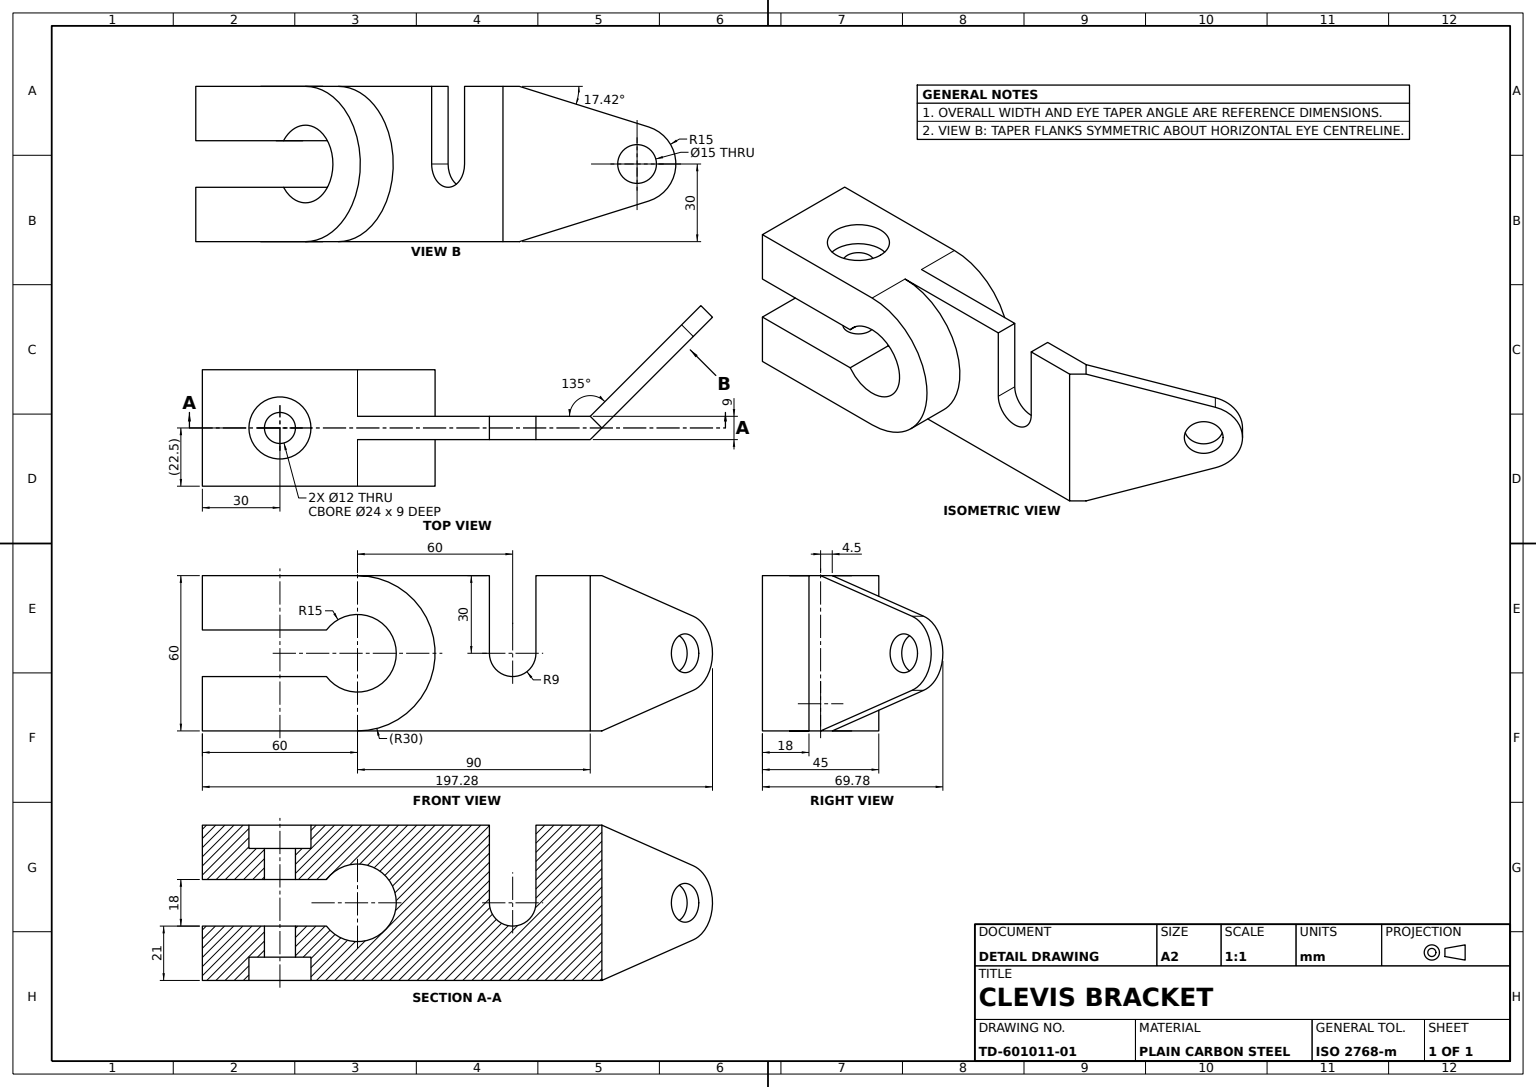
SolidWorks part; units mm, degrees
material "Plain Carbon Steel"
ref_plane "Front Plane" through (0, 0, 0) normal (0, 0, 1) x (1, 0, 0)
ref_plane "Top Plane" through (0, 0, 0) normal (0, 1, 0) x (1, 0, 0)
ref_plane "Right Plane" through (0, 0, 0) normal (1, 0, 0) x (0, 0, -1)
sketch "Clevis Block Sketch" plane through (0, 0, 0) normal (0, 0, 1) x (1, 0, 0)
  line L0 (0, -30) -> (-60, -30)
  line L5 (-60, -30) -> (-60, -9)
  line L6 (0, 30) -> (-60, 30)
  line L7 (0, 0) -> (-30, 0)
  line L8 (-12, 9) -> (-28.6182, 9)
  line L9 (-12, -9) -> (-28.6182, -9)
  line L10 (0, 9) -> (-30, 9) construction
  line L11 (0, -9) -> (-30, -9) construction
  line L12 (-28.6182, 9) -> (-60, 9)
  line L13 (-28.6182, -9) -> (-60, -9)
  line L14 (-60, 9) -> (-60, 30)
  arc A0 (-12, -9) -> (-12, 9) centre (0, 0) ccw
  arc A1 (0, -30) -> (0, 30) centre (0, 0) ccw
  dimension "D1" = 30
  dimension "D2" = 60
  dimension "D3" = 60
  dimension "D6" = 30
  dimension "D7" = 28.6182
  dimension "D4" = 9
  dimension "D5" = 9
extrude "Clevis Block" add sketch "Clevis Block Sketch" along normal mid plane 45 contours L0 A1 L6 L14 L12 L8 A0 L9 L13 L5
sketch "Counterbore Sketch" plane through (0, 30, 0) normal (0, 1, 0) x (1, 0, 0)
  line L0 (-30, 22.5) -> (-30, -22.5) construction
  line L1 (0, 22.5) -> (-60, 22.5) construction
  line L2 (0, -22.5) -> (-60, -22.5) construction
  circle A0 centre (-30, 0) radius 12
  dimension "D2" = 24
  dimension "D1" = 22.5
extrude "Pin Hole Counterbore" cut sketch "Counterbore Sketch" against normal blind 9
sketch "Pin Hole Sketch" plane through (0, 30, 0) normal (0, 1, 0) x (1, 0, 0)
  circle A0 centre (-30, 0) radius 6
  dimension "D1" = 12
extrude "Pin Hole Ø12" cut sketch "Pin Hole Sketch" against normal blind 21
mirror "Counterbore Mirror" about plane through (0, 0, 0) normal (0, 1, 0) of "Pin Hole Counterbore"
mirror "Pin Hole Mirror" about plane through (0, 0, 0) normal (0, 1, 0) of "Pin Hole Ø12"
sketch "Mounting Arm Sketch" plane through (0, 0, 0) normal (0, 1, 0) x (1, 0, 0)
  line L0 (0, 0) -> (90, 0) construction
  line L1 (0, -4.5) -> (90, -4.5)
  line L2 (0, 4.5) -> (90, 4.5)
  line L3 (90, -4.5) -> (137.28, 42.78)
  line L4 (137.28, 42.78) -> (132.78, 47.28)
  line L5 (132.78, 47.28) -> (90, 4.5)
  line L6 (0, -4.5) -> (0, 4.5)
  dimension "D3" = 90
  dimension "D4" = 135
  dimension "D5" = 135
  dimension "D6" = 60.5
  dimension "D1" = 4.5
  dimension "D2" = 4.5
extrude "Mounting Arm" add sketch "Mounting Arm Sketch" along normal mid plane 60
sketch "Arm Clearance Cut Sketch" plane through (0, 0, -4.5) normal (0, 0, -1) x (-1, 0, 0)
  line L0 (-51, 30) -> (-60, 30)
  line L1 (-90, 30) -> (0, 30) construction
  line L2 (-60, 30) -> (-60, 0) construction
  line L3 (-69, 30) -> (-51, 30)
  line L4 (-69, 30) -> (-69, 0)
  line L5 (-69, 39) -> (-69, 0) construction
  line L6 (-51, 21) -> (-51, 0)
  line L7 (0, 21) -> (-51, 21) construction
  line L8 (0, 39) -> (-69, 39) construction
  line L9 (-51, 21) -> (-51, 30)
  line L10 (-90, -30) -> (0, -30) construction
  line L11 (0, 30) -> (-60, 30) construction
  arc A0 (-69, 0) -> (-51, 0) centre (-60, 0) ccw
  line M5 (0, 30) -> (-90, 30)
  dimension "D1" = 60
  dimension "D4" = 30
  dimension "D2" = 9
extrude "Arm Clearance Cut" cut sketch "Arm Clearance Cut Sketch" against normal mid plane 60 contours L4 A0 L6 L9 M5
sketch "Eye Profile Cut Sketch" plane through (42.75, 0, 42.75) normal (-0.7071, 0, -0.7071) x (-0.7071, 0, 0.7071)
  line L0 (-66.8216, 0) -> (-127.3216, 0)
  line L1 (-66.8216, 30) -> (-66.8216, -30) construction
  line L2 (-127.3216, 30) -> (-127.3216, -30) construction
  line L3 (-127.3216, 30) -> (-127.3216, -30)
  line L6 (-66.8216, -30) -> (-116.8129, -14.3118)
  line L7 (-116.8129, 14.3118) -> (-66.8216, 30)
  line L8 (-66.8216, -30) -> (-127.3216, -30)
  line L9 (-127.3216, 30) -> (-66.8216, 30)
  line L10 (-66.8216, -30) -> (-127.3216, -30)
  line L11 (-127.3216, -30) -> (-127.3216, 30)
  line L12 (-66.8216, 30) -> (-127.3216, 30)
  circle A0 centre (-112.3216, 0) radius 7.5
  arc A2 (-116.8129, 14.3118) -> (-116.8129, -14.3118) centre (-112.3216, 0) ccw
  line M8 (-127.3216, -30) -> (-66.8216, -30)
  line M10 (-66.8216, 30) -> (-127.3216, 30)
  line M11 (-127.3216, 30) -> (-127.3216, -30)
  dimension "D2" = 15
  dimension "D3" = 30
  dimension "D1" = 45.5
extrude "Eye Profile Cut" cut sketch "Eye Profile Cut Sketch" against normal mid plane 60 contours A2 L7 M10 M11 | A2 L6 M11 M8
sketch "Eye Bore Sketch" plane through (42.75, 0, 42.75) normal (-0.7071, 0, -0.7071) x (-0.7071, 0, 0.7071)
  line L0 (-127.3216, 0) -> (-112.3216, 0) construction
  arc A0 (-116.8129, 14.3118) -> (-116.8129, -14.3118) centre (-112.3216, 0) ccw construction
  circle A1 centre (-112.3216, 0) radius 7.5
  dimension "D1" = 15
extrude "Eye Bore" cut sketch "Eye Bore Sketch" against normal mid plane 60
sketch "Relief Slot Sketch" plane through (0, 0, -22.5) normal (0, 0, -1) x (-1, 0, 0)
  line L0 (0, 15) -> (0, -15) construction
  line L1 (0, 15) -> (0, -15)
  arc A0 (12, 9) -> (12, -9) centre (0, 0) ccw construction
  arc A1 (0, 15) -> (0, -15) centre (0, 0) ccw
extrude "Relief Slot Cut" cut sketch "Relief Slot Sketch" against normal through all both and the other way through all
